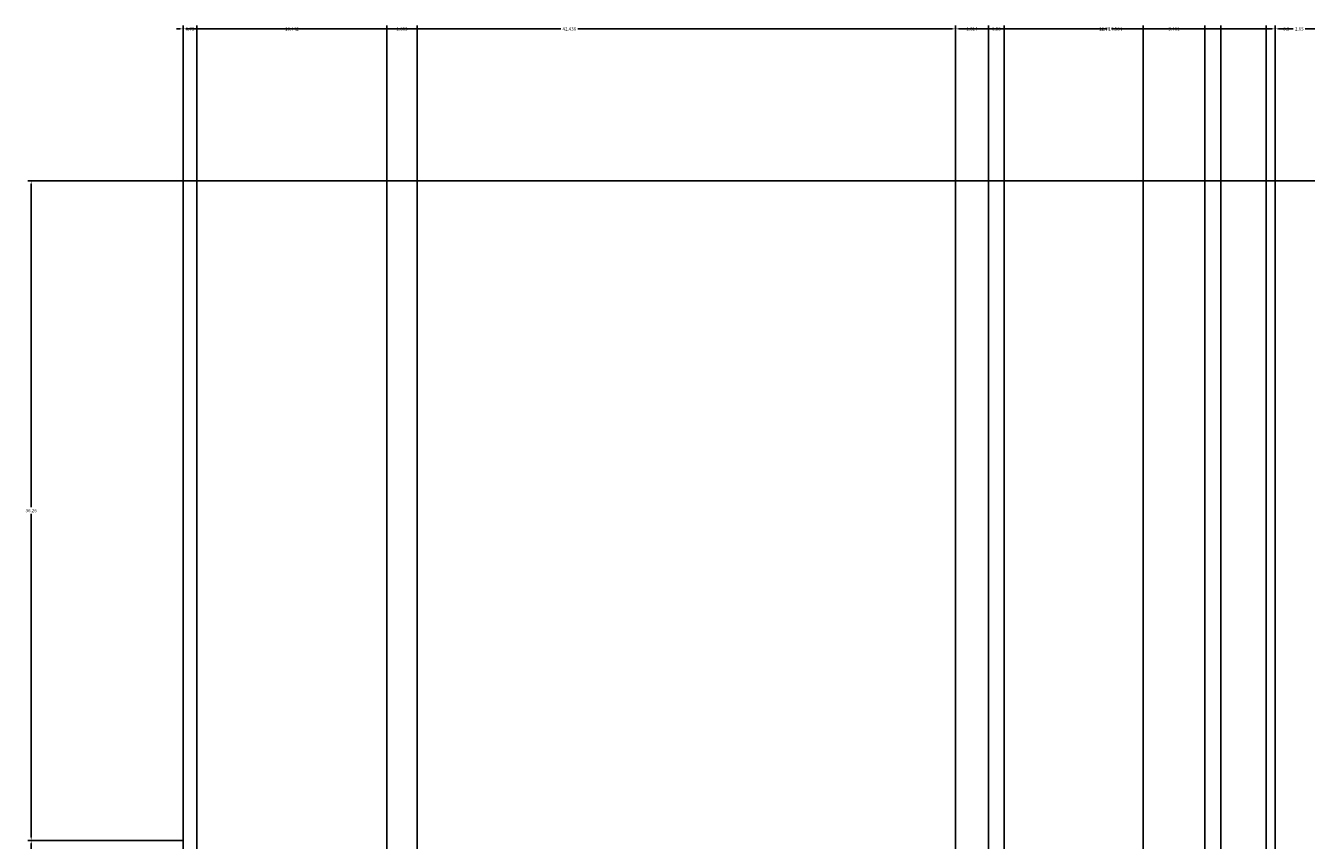
# Model space of a CAD drawing. Units: millimetres. Extents: x 446512 to 447461, y 70395 to 70610.
# Tile 20 of 39: x 446678 to 446748, y 70533 to 70578. Entities that reach past the tile are written whole.
import ezdxf

# ---------------------------------------------------------------- set-up
doc = ezdxf.new("R2010")
doc.units = ezdxf.units.MM
doc.layers.add('A-ANNO-DIMS', color=2, linetype='Continuous', lineweight=18)
doc.styles.get("Standard").update_dxf_attribs({"font": 'arial.ttf'})
doc.dimstyles.get("Standard").update_dxf_attribs({"dimtxt": 0.18, "dimasz": 0.18, "dimexe": 0.18, "dimexo": 0.0625, "dimgap": 0.09, "dimtad": 0, "dimtih": 1, "dimtoh": 1, "dimdec": 4, "dimzin": 0, "dimdsep": 46, "dimtxsty": 'Standard', "dimcen": 0.09, "dimadec": 0, "dimazin": 0, "dimtfac": 1, "dimtdec": 4, "dimtofl": 0, "dimtmove": 0, "dimatfit": 3, "dimfxl": 1, "dimtolj": 1, "dimtzin": 0, "dimarcsym": 0})

# ---------------------------------------------------------------- blocks, each defined once
blk = doc.blocks.new('*D13')
at = {"layer": 'A-ANNO-DIMS', "color": 0, "lineweight": -2, "transparency": 16777216}
for p, q in [((446686.573, 70533.444), (446686.573, 70578.175)), ((446686.753, 70577.995), (446707.323, 70577.995)), ((446728.828, 70577.995), (446708.258, 70577.995)), ((446729.008, 70533.444), (446729.008, 70578.175))]:
    blk.add_line(p, q, dxfattribs=at)
at = {"layer": 'A-ANNO-DIMS', "color": 0, "transparency": 16777216}
for points in [[(446686.753, 70578.025), (446686.753, 70577.965), (446686.573, 70577.995)], [(446728.828, 70578.025), (446728.828, 70577.965), (446729.008, 70577.995)]]:
    blk.add_solid(points, dxfattribs=at)
at = {"layer": 'Defpoints', "color": 0, "transparency": 16777216}
for p in [(446729.008, 70577.995), (446686.573, 70533.382), (446729.008, 70533.382)]:
    blk.add_point(p, dxfattribs=at)
at = {"layer": 'A-ANNO-DIMS', "color": 0, "transparency": 16777216, "insert": (446707.791, 70577.995), "char_height": 0.18, "attachment_point": 5}
blk.add_mtext('\\A1;42.436', dxfattribs=at)
blk = doc.blocks.new('*D14')
at = {"layer": 'A-ANNO-DIMS', "color": 0, "lineweight": -2, "transparency": 16777216}
for p, q in [((446729.008, 70533.444), (446729.008, 70578.175)), ((446729.188, 70577.995), (446737.336, 70577.995)), ((446746.393, 70577.995), (446738.245, 70577.995)), ((446746.573, 70533.444), (446746.573, 70578.175))]:
    blk.add_line(p, q, dxfattribs=at)
at = {"layer": 'A-ANNO-DIMS', "color": 0, "transparency": 16777216}
for points in [[(446729.188, 70578.025), (446729.188, 70577.965), (446729.008, 70577.995)], [(446746.393, 70578.025), (446746.393, 70577.965), (446746.573, 70577.995)]]:
    blk.add_solid(points, dxfattribs=at)
at = {"layer": 'Defpoints', "color": 0, "transparency": 16777216}
for p in [(446746.573, 70577.995), (446729.008, 70533.382), (446746.573, 70533.382)]:
    blk.add_point(p, dxfattribs=at)
at = {"layer": 'A-ANNO-DIMS', "color": 0, "transparency": 16777216, "insert": (446737.791, 70577.995), "char_height": 0.18, "attachment_point": 5}
blk.add_mtext('\\A1;17.564', dxfattribs=at)
blk = doc.blocks.new('*D15')
at = {"layer": 'A-ANNO-DIMS', "color": 0, "lineweight": -2, "transparency": 16777216}
for p, q in [((446746.573, 70533.444), (446746.573, 70578.175)), ((446746.753, 70577.995), (446747.572, 70577.995)), ((446749.043, 70577.995), (446748.224, 70577.995)), ((446749.223, 70569.707), (446749.223, 70578.175))]:
    blk.add_line(p, q, dxfattribs=at)
at = {"layer": 'A-ANNO-DIMS', "color": 0, "transparency": 16777216}
for points in [[(446746.753, 70578.025), (446746.753, 70577.965), (446746.573, 70577.995)], [(446749.043, 70578.025), (446749.043, 70577.965), (446749.223, 70577.995)]]:
    blk.add_solid(points, dxfattribs=at)
at = {"layer": 'Defpoints', "color": 0, "transparency": 16777216}
for p in [(446749.223, 70577.995), (446749.223, 70569.645), (446746.573, 70533.382)]:
    blk.add_point(p, dxfattribs=at)
at = {"layer": 'A-ANNO-DIMS', "color": 0, "transparency": 16777216, "insert": (446747.898, 70577.995), "char_height": 0.18, "attachment_point": 5}
blk.add_mtext('\\A1;2.65', dxfattribs=at)
blk = doc.blocks.new('*D23')
at = {"layer": 'A-ANNO-DIMS', "color": 0, "lineweight": -2, "transparency": 16777216}
for p, q in [((446686.51, 70533.382), (446678.043, 70533.382)), ((446678.223, 70533.202), (446678.223, 70523.563)), ((446678.223, 70513.562), (446678.223, 70523.2)), ((446686.51, 70513.382), (446678.043, 70513.382))]:
    blk.add_line(p, q, dxfattribs=at)
at = {"layer": 'A-ANNO-DIMS', "color": 0, "transparency": 16777216}
for points in [[(446678.193, 70533.202), (446678.253, 70533.202), (446678.223, 70533.382)], [(446678.193, 70513.562), (446678.253, 70513.562), (446678.223, 70513.382)]]:
    blk.add_solid(points, dxfattribs=at)
at = {"layer": 'Defpoints', "color": 0, "transparency": 16777216}
for p in [(446678.223, 70533.382), (446686.573, 70533.382), (446686.573, 70513.382)]:
    blk.add_point(p, dxfattribs=at)
at = {"layer": 'A-ANNO-DIMS', "color": 0, "transparency": 16777216, "insert": (446678.223, 70523.382), "char_height": 0.18, "attachment_point": 5}
blk.add_mtext('\\A1;20', dxfattribs=at)
blk = doc.blocks.new('*D24')
at = {"layer": 'A-ANNO-DIMS', "color": 0, "lineweight": -2, "transparency": 16777216}
for p, q in [((446749.161, 70569.645), (446678.043, 70569.645)), ((446678.223, 70569.465), (446678.223, 70551.695)), ((446678.223, 70533.562), (446678.223, 70551.331)), ((446686.51, 70533.382), (446678.043, 70533.382))]:
    blk.add_line(p, q, dxfattribs=at)
at = {"layer": 'A-ANNO-DIMS', "color": 0, "transparency": 16777216}
for points in [[(446678.193, 70569.465), (446678.253, 70569.465), (446678.223, 70569.645)], [(446678.193, 70533.562), (446678.253, 70533.562), (446678.223, 70533.382)]]:
    blk.add_solid(points, dxfattribs=at)
at = {"layer": 'Defpoints', "color": 0, "transparency": 16777216}
for p in [(446678.223, 70569.645), (446749.223, 70569.645), (446686.573, 70533.382)]:
    blk.add_point(p, dxfattribs=at)
at = {"layer": 'A-ANNO-DIMS', "color": 0, "transparency": 16777216, "insert": (446678.223, 70551.513), "char_height": 0.18, "attachment_point": 5}
blk.add_mtext('\\A1;36.26', dxfattribs=at)
blk = doc.blocks.new('*D29')
at = {"layer": 'A-ANNO-DIMS', "color": 0, "lineweight": -2, "transparency": 16777216}
for p, q in [((446730.822, 70489.647), (446730.822, 70578.175)), ((446731.002, 70577.995), (446736.817, 70577.995)), ((446743.402, 70577.995), (446737.587, 70577.995)), ((446743.582, 70489.647), (446743.582, 70578.175))]:
    blk.add_line(p, q, dxfattribs=at)
at = {"layer": 'A-ANNO-DIMS', "color": 0, "transparency": 16777216}
for points in [[(446731.002, 70578.025), (446731.002, 70577.965), (446730.822, 70577.995)], [(446743.402, 70578.025), (446743.402, 70577.965), (446743.582, 70577.995)]]:
    blk.add_solid(points, dxfattribs=at)
at = {"layer": 'Defpoints', "color": 0, "transparency": 16777216}
for p in [(446743.582, 70577.995), (446730.822, 70489.584), (446743.582, 70489.584)]:
    blk.add_point(p, dxfattribs=at)
at = {"layer": 'A-ANNO-DIMS', "color": 0, "transparency": 16777216, "insert": (446737.202, 70577.995), "char_height": 0.18, "attachment_point": 5}
blk.add_mtext('\\A1;12.76', dxfattribs=at)
blk = doc.blocks.new('*D31')
at = {"layer": 'A-ANNO-DIMS', "color": 0, "lineweight": -2, "transparency": 16777216}
for p, q in [((446729.008, 70473.444), (446729.008, 70578.175)), ((446729.188, 70577.995), (446729.531, 70577.995)), ((446730.642, 70577.995), (446730.3, 70577.995)), ((446730.822, 70474.467), (446730.822, 70578.175))]:
    blk.add_line(p, q, dxfattribs=at)
at = {"layer": 'A-ANNO-DIMS', "color": 0, "transparency": 16777216}
for points in [[(446729.188, 70578.025), (446729.188, 70577.965), (446729.008, 70577.995)], [(446730.642, 70578.025), (446730.642, 70577.965), (446730.822, 70577.995)]]:
    blk.add_solid(points, dxfattribs=at)
at = {"layer": 'Defpoints', "color": 0, "transparency": 16777216}
for p in [(446730.822, 70577.995), (446730.822, 70474.405), (446729.008, 70473.382)]:
    blk.add_point(p, dxfattribs=at)
at = {"layer": 'A-ANNO-DIMS', "color": 0, "transparency": 16777216, "insert": (446729.915, 70577.995), "char_height": 0.18, "attachment_point": 5}
blk.add_mtext('\\A1;1.814', dxfattribs=at)
blk = doc.blocks.new('*D33')
at = {"layer": 'A-ANNO-DIMS', "color": 0, "lineweight": -2, "transparency": 16777216}
for p, q in [((446730.642366, 70577.99492), (446730.462366, 70577.99492)), ((446730.822366, 70489.64696), (446730.822366, 70578.17492)), ((446731.68472, 70488.784606), (446731.68472, 70578.17492)), ((446731.86472, 70577.99492), (446732.04472, 70577.99492))]:
    blk.add_line(p, q, dxfattribs=at)
at = {"layer": 'A-ANNO-DIMS', "color": 0, "transparency": 16777216}
for points in [[(446730.642366, 70578.02492), (446730.642366, 70577.96492), (446730.822366, 70577.99492)], [(446731.86472, 70578.02492), (446731.86472, 70577.96492), (446731.68472, 70577.99492)]]:
    blk.add_solid(points, dxfattribs=at)
at = {"layer": 'Defpoints', "color": 0, "transparency": 16777216}
for p in [(446731.68472, 70577.99492), (446730.822366, 70489.58446), (446731.68472, 70488.722106)]:
    blk.add_point(p, dxfattribs=at)
at = {"layer": 'A-ANNO-DIMS', "color": 0, "transparency": 16777216, "insert": (446731.253543, 70577.99492), "char_height": 0.18, "attachment_point": 5}
blk.add_mtext('\\A1;0.86', dxfattribs=at)
blk = doc.blocks.new('*D34')
at = {"layer": 'A-ANNO-DIMS', "color": 0, "lineweight": -2, "transparency": 16777216}
for p, q in [((446739.318, 70485.567), (446739.318, 70578.175)), ((446739.498, 70577.995), (446740.642, 70577.995)), ((446742.539, 70577.995), (446741.395, 70577.995)), ((446742.719, 70488.785), (446742.719, 70578.175))]:
    blk.add_line(p, q, dxfattribs=at)
at = {"layer": 'A-ANNO-DIMS', "color": 0, "transparency": 16777216}
for points in [[(446739.498, 70578.025), (446739.498, 70577.965), (446739.318, 70577.995)], [(446742.539, 70578.025), (446742.539, 70577.965), (446742.719, 70577.995)]]:
    blk.add_solid(points, dxfattribs=at)
at = {"layer": 'Defpoints', "color": 0, "transparency": 16777216}
for p in [(446739.318, 70577.995), (446742.719, 70488.722), (446739.318, 70485.504)]:
    blk.add_point(p, dxfattribs=at)
at = {"layer": 'A-ANNO-DIMS', "color": 0, "transparency": 16777216, "insert": (446741.019, 70577.995), "char_height": 0.18, "attachment_point": 5}
blk.add_mtext('\\A1;3.401', dxfattribs=at)
blk = doc.blocks.new('*D36')
at = {"layer": 'A-ANNO-DIMS', "color": 0, "lineweight": -2, "transparency": 16777216}
for p, q in [((446745.893, 70577.995), (446745.713, 70577.995)), ((446746.073, 70472.944), (446746.073, 70578.175)), ((446746.573, 70473.444), (446746.573, 70578.175)), ((446746.753, 70577.995), (446746.933, 70577.995))]:
    blk.add_line(p, q, dxfattribs=at)
at = {"layer": 'A-ANNO-DIMS', "color": 0, "transparency": 16777216}
for points in [[(446745.893, 70578.025), (446745.893, 70577.965), (446746.073, 70577.995)], [(446746.753, 70578.025), (446746.753, 70577.965), (446746.573, 70577.995)]]:
    blk.add_solid(points, dxfattribs=at)
at = {"layer": 'Defpoints', "color": 0, "transparency": 16777216}
for p in [(446746.573, 70577.995), (446746.573, 70473.382), (446746.073, 70472.882)]:
    blk.add_point(p, dxfattribs=at)
at = {"layer": 'A-ANNO-DIMS', "color": 0, "transparency": 16777216, "insert": (446747.187, 70577.995), "char_height": 0.18, "attachment_point": 5}
blk.add_mtext('\\A1;0.5', dxfattribs=at)
blk = doc.blocks.new('*D37')
at = {"layer": 'A-ANNO-DIMS', "color": 0, "lineweight": -2, "transparency": 16777216}
for p, q in [((446686.392846, 70577.99492), (446686.212846, 70577.99492)), ((446686.572846, 70433.44405), (446686.572846, 70578.17492)), ((446687.323552, 70428.838404), (446687.323552, 70578.17492)), ((446687.503552, 70577.99492), (446687.683552, 70577.99492))]:
    blk.add_line(p, q, dxfattribs=at)
at = {"layer": 'A-ANNO-DIMS', "color": 0, "transparency": 16777216}
for points in [[(446686.392846, 70578.02492), (446686.392846, 70577.96492), (446686.572846, 70577.99492)], [(446687.503552, 70578.02492), (446687.503552, 70577.96492), (446687.323552, 70577.99492)]]:
    blk.add_solid(points, dxfattribs=at)
at = {"layer": 'Defpoints', "color": 0, "transparency": 16777216}
for p in [(446687.323552, 70577.99492), (446686.572846, 70433.38155), (446687.323552, 70428.775904)]:
    blk.add_point(p, dxfattribs=at)
at = {"layer": 'A-ANNO-DIMS', "color": 0, "transparency": 16777216, "insert": (446686.948199, 70577.99492), "char_height": 0.18, "attachment_point": 5}
blk.add_mtext('\\A1;0.75', dxfattribs=at)
blk = doc.blocks.new('*D38')
at = {"layer": 'A-ANNO-DIMS', "color": 0, "lineweight": -2, "transparency": 16777216}
for p, q in [((446687.323552, 70428.838404), (446687.323552, 70578.17492)), ((446687.503552, 70577.99492), (446692.090383, 70577.99492)), ((446697.585686, 70577.99492), (446692.998855, 70577.99492)), ((446697.765686, 70428.838404), (446697.765686, 70578.17492))]:
    blk.add_line(p, q, dxfattribs=at)
at = {"layer": 'A-ANNO-DIMS', "color": 0, "transparency": 16777216}
for points in [[(446687.503552, 70578.02492), (446687.503552, 70577.96492), (446687.323552, 70577.99492)], [(446697.585686, 70578.02492), (446697.585686, 70577.96492), (446697.765686, 70577.99492)]]:
    blk.add_solid(points, dxfattribs=at)
at = {"layer": 'Defpoints', "color": 0, "transparency": 16777216}
for p in [(446697.765686, 70577.99492), (446687.323552, 70428.775904), (446697.765686, 70428.775904)]:
    blk.add_point(p, dxfattribs=at)
at = {"layer": 'A-ANNO-DIMS', "color": 0, "transparency": 16777216, "insert": (446692.544619, 70577.99492), "char_height": 0.18, "attachment_point": 5}
blk.add_mtext('\\A1;10.442', dxfattribs=at)
blk = doc.blocks.new('*D39')
at = {"layer": 'A-ANNO-DIMS', "color": 0, "lineweight": -2, "transparency": 16777216}
for p, q in [((446697.766, 70428.838), (446697.766, 70578.175)), ((446697.946, 70577.995), (446698.212, 70577.995)), ((446699.249, 70577.995), (446698.982, 70577.995)), ((446699.429, 70433.444), (446699.429, 70578.175))]:
    blk.add_line(p, q, dxfattribs=at)
at = {"layer": 'A-ANNO-DIMS', "color": 0, "transparency": 16777216}
for points in [[(446697.946, 70578.025), (446697.946, 70577.965), (446697.766, 70577.995)], [(446699.249, 70578.025), (446699.249, 70577.965), (446699.429, 70577.995)]]:
    blk.add_solid(points, dxfattribs=at)
at = {"layer": 'Defpoints', "color": 0, "transparency": 16777216}
for p in [(446699.429, 70577.995), (446699.429, 70433.382), (446697.766, 70428.776)]:
    blk.add_point(p, dxfattribs=at)
at = {"layer": 'A-ANNO-DIMS', "color": 0, "transparency": 16777216, "insert": (446698.597, 70577.995), "char_height": 0.18, "attachment_point": 5}
blk.add_mtext('\\A1;1.663', dxfattribs=at)

msp = doc.modelspace()

# ---------------------------------------------------------------- dimensions: what is measured, and where the dimension line sits
at = {"layer": 'A-ANNO-DIMS'}
for base, p1, p2, override, picture, middle in [((446687.3236, 70577.9949), (446686.5728, 70433.3816), (446687.3236, 70428.7759), {"dimdec": 2, "dimlfac": 1, "dimrnd": 0, "dimzin": 0, "dimdsep": 46, "dimlunit": 2}, '*D37', (446686.9482, 70577.9949)), ((446729.0084, 70577.9949), (446686.5728, 70533.3816), (446729.0084, 70533.3816), {"dimdec": 3, "dimlfac": 1, "dimrnd": 0, "dimzin": 0, "dimdsep": 46, "dimlunit": 2}, '*D13', (446707.7906, 70577.9949)), ((446697.7657, 70577.9949), (446687.3236, 70428.7759), (446697.7657, 70428.7759), {"dimdec": 3, "dimlfac": 1, "dimrnd": 0, "dimzin": 0, "dimdsep": 46, "dimlunit": 2}, '*D38', (446692.5446, 70577.9949)), ((446699.4288, 70577.9949), (446697.7657, 70428.7759), (446699.4288, 70433.3816), {"dimdec": 3, "dimlfac": 1, "dimrnd": 0, "dimzin": 0, "dimdsep": 46, "dimlunit": 2}, '*D39', (446698.5973, 70577.9949)), ((446746.5728, 70577.9949), (446729.0084, 70533.3816), (446746.5728, 70533.3816), {"dimdec": 3, "dimlfac": 1, "dimrnd": 0, "dimzin": 0, "dimdsep": 46, "dimlunit": 2}, '*D14', (446737.7906, 70577.9949)), ((446730.8224, 70577.9949), (446729.0084, 70473.3816), (446730.8224, 70474.4047), {"dimdec": 3, "dimlfac": 1, "dimrnd": 0, "dimzin": 0, "dimdsep": 46, "dimlunit": 2}, '*D31', (446729.9154, 70577.9949)), ((446731.6847, 70577.9949), (446730.8224, 70489.5845), (446731.6847, 70488.7221), {"dimdec": 2, "dimlfac": 1, "dimrnd": 0, "dimzin": 0, "dimdsep": 46, "dimlunit": 2}, '*D33', (446731.2535, 70577.9949)), ((446743.5815, 70577.9949), (446730.8224, 70489.5845), (446743.5815, 70489.5845), {"dimdec": 2, "dimlfac": 1, "dimrnd": 0, "dimzin": 0, "dimdsep": 46, "dimlunit": 2}, '*D29', (446737.2019, 70577.9949)), ((446739.3181, 70577.9949), (446742.7192, 70488.7221), (446739.3181, 70485.5045), {"dimdec": 3, "dimlfac": 1, "dimrnd": 0, "dimzin": 0, "dimdsep": 46, "dimlunit": 2}, '*D34', (446741.0186, 70577.9949)), ((446746.5728, 70577.9949), (446746.0728, 70472.8816), (446746.5728, 70473.3816), {"dimdec": 1, "dimlfac": 1, "dimrnd": 0, "dimzin": 0, "dimdsep": 46, "dimlunit": 2}, '*D36', (446747.1874, 70577.9949)), ((446749.2235, 70577.9949), (446746.5728, 70533.3816), (446749.2235, 70569.6449), {"dimdec": 2, "dimlfac": 1, "dimrnd": 0, "dimzin": 0, "dimdsep": 46, "dimlunit": 2}, '*D15', (446747.8982, 70577.9949))]:
    dim = msp.add_linear_dim(base=base, p1=p1, p2=p2, dimstyle='Standard', override=override, dxfattribs=at)
    dim.commit()
    dim.dimension.update_dxf_attribs({"geometry": picture, "text_midpoint": middle})
for base, p1, p2, override, picture, middle in [((446678.2228, 70569.6449), (446686.5728, 70533.3816), (446749.2235, 70569.6449), {"dimdec": 2, "dimlfac": 1, "dimrnd": 0, "dimzin": 0, "dimdsep": 46, "dimlunit": 2}, '*D24', (446678.2228, 70551.5132)), ((446678.2228, 70533.3816), (446686.5728, 70513.3816), (446686.5728, 70533.3816), {"dimdec": 0, "dimlfac": 1, "dimrnd": 0, "dimzin": 0, "dimdsep": 46, "dimlunit": 2}, '*D23', (446678.2228, 70523.3815))]:
    dim = msp.add_linear_dim(base=base, p1=p1, p2=p2, angle=90, dimstyle='Standard', override=override, dxfattribs=at)
    dim.commit()
    dim.dimension.update_dxf_attribs({"geometry": picture, "text_midpoint": middle})

doc.saveas('drawing.dxf')
